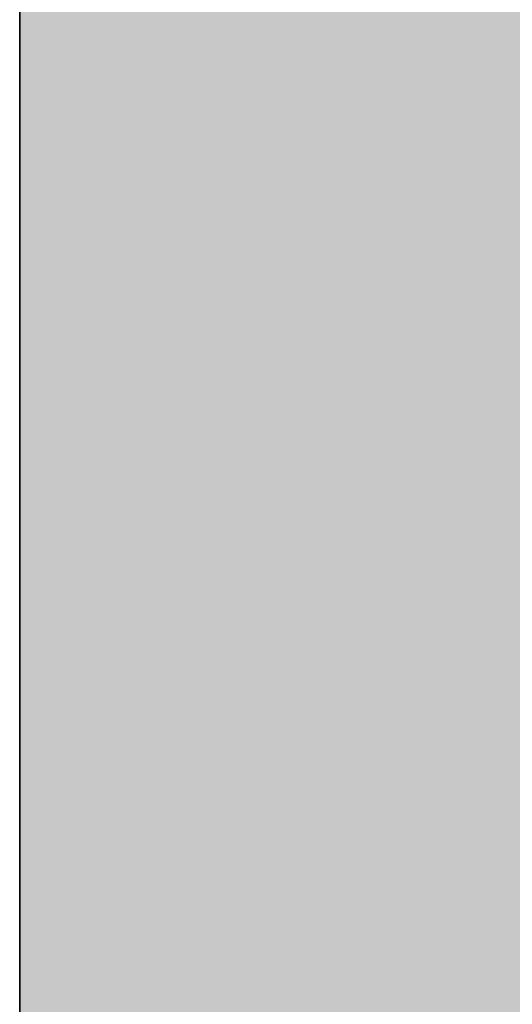
# Model space of a CAD drawing. Units: inches. Extents: x 2091 to 2899, y 967 to 2217.
# Tile 163 of 256: x 2203.143603 to 2203.144443, y 1152.248741 to 1152.250422. Entities that reach past the tile are written whole.
import ezdxf

# ---------------------------------------------------------------- set-up
doc = ezdxf.new("R2010")
doc.units = ezdxf.units.IN
doc.layers.add('A-WALL-PATT', color=141, linetype='Continuous', lineweight=13, true_color=0xadddf7)
doc.layers.add('C-PROP', color=7, linetype='Continuous', lineweight=35)

msp = doc.modelspace()

# ---------------------------------------------------------------- hatches: boundary and pattern name
at = {"layer": 'A-WALL-PATT'}
h = msp.add_hatch(color=256, dxfattribs=at)
h.dxf.hatch_style = 1
h.paths.add_polyline_path([(2803.1436027, 2050.9190588), (2203.1436027, 2050.9190588), (2203.1436027, 1090.9190588), (2803.1436027, 1090.9190588)])
h.paths.add_polyline_path([(2635.7988501, 1147.5404649), (2674.5240524, 1147.5404649, 0.376086), (2678.5296653, 1152.8802017), (2678.5296653, 1159.5564734, 0.333335), (2674.524319, 1163.561846), (2674.524319, 1163.5618504), (2674.524319, 1192.9343904), (2635.8059707, 1192.9343904), (2597.0876225, 1192.9343904), (2597.0876225, 1163.561846, 0.333335), (2593.0822761, 1159.5564734), (2593.0822761, 1152.8802017, 0.376086), (2597.087889, 1147.5404649)], flags=0)
h.paths.add_polyline_path([(2436.0104329, 1278.2407784, 0.000483), (2435.9526433, 1278.215027, -0.001328), (2435.9356253, 1278.1116934, -0.001711), (2436.1164401, 1278.0407583, 0.002185)], flags=0)
h.paths.add_polyline_path([(2794.1436027, 1143.4190588), (2794.1436027, 1347.4190588), (2543.3701706, 1347.4190588), (2543.3701706, 1351.9190588), (2794.1436027, 1351.9190588), (2794.1436027, 1392.7135549), (2793.9473982, 1392.7135549), (2793.9473982, 1473.5368999), (2794.1436027, 1473.5368999), (2794.1436027, 1531.9190588), (2650.1436027, 1531.9190588), (2650.1436027, 1536.4190588), (2794.1436027, 1536.4190588), (2794.1436027, 1692.4190588), (2609.3756095, 1692.4190588), (2609.3756095, 1644.4190588), (2604.8756095, 1644.4190588), (2604.8756095, 1744.9190588), (2609.3756095, 1744.9190588), (2609.3756095, 1696.9190588), (2794.1436027, 1696.9190588), (2794.1436027, 1780.9190588), (2609.6436027, 1780.9190588), (2493.8756095, 1780.9190588), (2493.8756095, 1785.4190588), (2609.6436027, 1785.4190588), (2794.1436027, 1785.4190588), (2794.1436027, 1847.9388214), (2793.9512217, 1847.9388214), (2793.9512217, 1928.7621663), (2794.1436027, 1928.7621663), (2794.1436027, 1941.4190588), (2614.1436027, 1941.4190588), (2614.1436027, 1821.4190588), (2609.6436027, 1821.4190588), (2609.6436027, 1941.4190588), (2392.1436027, 1941.4190588), (2392.1436027, 1819.9190588), (2387.6436027, 1819.9190588), (2387.6436027, 1941.4190588), (2212.1436027, 1941.4190588), (2212.1436027, 1783.9190588), (2392.1436027, 1783.9190588), (2392.1436027, 1780.9190588), (2212.1436027, 1780.9190588), (2212.1436027, 1629.4190588), (2387.6436027, 1629.4190588), (2387.6436027, 1744.9190588), (2392.1436027, 1744.9190588), (2392.1436027, 1627.9190588), (2317.1436027, 1627.9190588), (2317.1436027, 1551.4190588), (2317.1436027, 1536.4190588), (2459.3835909, 1536.4190588), (2459.3835909, 1602.3964802), (2463.8835909, 1602.3964802), (2463.8835909, 1531.9190588), (2456.6436027, 1531.9190588), (2456.6436027, 1529.9190588), (2452.1436027, 1529.9190588), (2452.1436027, 1531.9190588), (2312.6436027, 1531.9190588), (2312.6436027, 1551.4190588), (2306.1436027, 1551.4190588), (2306.1436027, 1555.9190588), (2308.1436027, 1555.9190588), (2308.1436027, 1551.4190588), (2312.6436027, 1551.4190588), (2312.6436027, 1627.9190588), (2212.1436027, 1627.9190588), (2212.1436027, 1555.9190588), (2270.1436027, 1555.9190588), (2270.1436027, 1551.4190588), (2212.1436027, 1551.4190588), (2212.1436027, 1351.9190588), (2272.1436027, 1351.9190588), (2272.1436027, 1347.4190588), (2212.1436027, 1347.4190588), (2212.1436027, 1275.4190588), (2308.1436027, 1275.4190588), (2308.1436027, 1351.9190588), (2452.1436027, 1351.9190588), (2452.1436027, 1493.9190588), (2456.6436027, 1493.9190588), (2456.6436027, 1347.4190588), (2312.6436027, 1347.4190588), (2312.6436027, 1270.9190588), (2212.1436027, 1270.9190588), (2212.1436027, 1099.9190588), (2281.2375229, 1099.9190588), (2282.8710413, 1110.9138034), (2282.0083413, 1116.9966034), (2278.5577413, 1121.4204034), (2268.2056413, 1128.0562034), (2272.0876413, 1128.0562034), (2273.8129413, 1131.9270034), (2279.4203413, 1134.6919034), (2285.0278413, 1135.2449034), (2287.6158413, 1137.4568034), (2288.0471413, 1138.0098034), (2289.3411413, 1140.7747034), (2291.0665413, 1139.6687034), (2292.3605413, 1135.2449034), (2295.3798413, 1136.9038034), (2296.2425413, 1135.7979034), (2297.1052413, 1133.0330034), (2300.1246413, 1138.0098034), (2303.1439413, 1138.0098034), (2304.4379413, 1135.7979034), (2303.1439413, 1133.5860034), (2306.5946413, 1134.6919034), (2307.8887413, 1133.0330034), (2310.9080413, 1135.2449034), (2313.9274413, 1134.1389034), (2315.6268599, 1132.4271023), (2308.3200413, 1117.5496034), (2290.2038413, 1109.8079034), (2288.9098413, 1103.1721034), (2289.2723086, 1099.9190588), (2434.9182274, 1099.9190588), (2431.5932274, 1124.7880588), (2429.9302274, 1169.5530588), (2430.9271848, 1240.5196942), (2435.6589255, 1238.1861258), (2437.1352274, 1196.5540588), (2438.7982274, 1143.9730588), (2442.6782274, 1111.9980588), (2446.5582274, 1099.9190588), (2794.1436027, 1099.9190588), (2794.1436027, 1138.9190588), (2548.0324471, 1138.9190588), (2548.0324471, 1143.4190588), (2548.0324471, 1148.8190588), (2546.6684571, 1148.0315588), (2528.6856919, 1179.1786218, 0.256256), (2512.0324471, 1148.8190588), (2512.0324471, 1143.4190588), (2512.0324471, 1138.9190588), (2507.5324471, 1138.9190588), (2507.5324471, 1143.4190588), (2507.5324471, 1148.8190588, 0.256256), (2490.8792023, 1179.1786218), (2472.8964371, 1148.0315588), (2471.5324471, 1148.8190588), (2471.5324471, 1143.4190588), (2467.0324471, 1143.4190588), (2467.0324471, 1269.9457858, 0.039061), (2460.9099871, 1273.5800588), (2467.0324471, 1273.5800588), (2467.0324471, 1286.3253638, 0.014511), (2465.2161944, 1286.7619052), (2467.0324471, 1287.0525761), (2467.0324471, 1323.4190588), (2471.5324471, 1323.4190588), (2471.5324471, 1148.8190588), (2489.5324471, 1179.9959734), (2490.8964371, 1179.2084734), (2490.8792023, 1179.1786218, -0.256256), (2507.5324471, 1148.8190588), (2507.5324471, 1143.4190588), (2512.0324471, 1143.4190588), (2512.0324471, 1148.8190588, -0.256256), (2528.6856919, 1179.1786218), (2528.6684571, 1179.2084734), (2530.0324471, 1179.9959734), (2548.0324471, 1148.8190588), (2548.0324471, 1143.4190588)], flags=16)
h.paths.add_polyline_path([(2607.7685461, 1200.9450832), (2607.7685461, 1265.0306251), (2597.0876225, 1281.0520106), (2619.7845852, 1281.0520106), (2627.795278, 1337.1268598), (2635.7988501, 1337.1268598), (2643.8166634, 1337.1268598), (2651.8273562, 1281.0520106), (2674.524319, 1281.0520106), (2663.8433953, 1265.0306251), (2663.8433953, 1200.9450832), (2635.8059707, 1200.9450832)], flags=0)
edge = h.paths.add_edge_path(flags=0)
edge.add_ellipse((13303.8962153, 1272.9987247), major_axis=(-10595.3130399, 0.0000005), ratio=0.842303870086, start_angle=0.62823721906, end_angle=0.64655409989, ccw=False)
edge.add_ellipse((2711.7004495, 1156.8526781), major_axis=(2.2197691, 0), ratio=0.84230387, start_angle=111.5352435, end_angle=180.6282372, ccw=False)
edge.add_ellipse((13303.1562922, 1272.9987246), major_axis=(-10593.0263064, 0), ratio=0.842303869544, start_angle=0.52827147182, end_angle=0.64655409706, ccw=False)
edge.add_line((2710.7645961, 1175.3332951), (2710.1299858, 1175.3332951))
edge.add_ellipse((2710.1299858, 1176.5797752), major_axis=(1.4798461, 0), ratio=0.84230387, start_angle=180, end_angle=270, ccw=False)
edge.add_line((2708.6501397, 1176.5797752), (2708.6501397, 1200.7829144))
edge.add_ellipse((2710.1299858, 1200.7829144), major_axis=(1.4798461, 0), ratio=0.84230387, start_angle=90, end_angle=180, ccw=False)
edge.add_line((2710.1299858, 1202.0293944), (2710.4650752, 1202.0293944))
edge.add_ellipse((13303.1562922, 1272.9987246), major_axis=(-10593.0263064, 0), ratio=0.842303869544, start_angle=-0.09022908859, end_angle=0.38386677879, ccw=False)
edge.add_ellipse((2710.1299858, 1290.9270308), major_axis=(-1.4798461, 0), ratio=0.84230387, start_angle=0, end_angle=90, ccw=False)
edge.add_line((2708.6501397, 1290.9270308), (2708.6501397, 1315.13017))
edge.add_ellipse((2710.1299858, 1315.13017), major_axis=(-1.4798461, 0), ratio=0.84230387, start_angle=-90, end_angle=0, ccw=False)
edge.add_line((2710.1299858, 1316.3766501), (2710.7063141, 1316.3766501))
edge.add_ellipse((3238.4017202, 1296.2895655), major_axis=(528.2339998, 0), ratio=0.84230386954, start_angle=176.349572414, end_angle=177.820049686, ccw=False)
edge.add_ellipse((2775.0630432, 1071.4506962), major_axis=(313.3077613, 0), ratio=0.84230386954, start_angle=102.125965552, end_angle=103.780528989, ccw=False)
edge.add_ellipse((2775.0630432, 1078.3056979), major_axis=(-305.3028915, 0), ratio=0.84230386955, start_angle=-79.790461003, end_angle=-77.555372706, ccw=False)
edge.add_ellipse((2695.1417666, 1541.9753825), major_axis=(-250.9602162, 0), ratio=0.84230386954, start_angle=99.256566007, end_angle=102.554932644)
edge.add_line((2741.4103262, 1334.2142554), (2747.1325454, 1337.3784768))
edge.add_ellipse((2747.5386163, 1336.8574776), major_axis=(-0.739923, 0), ratio=0.84230387, start_angle=270, end_angle=307.9331305, ccw=False)
edge.add_ellipse((2747.5386163, 1336.8574776), major_axis=(-0.739923, 0), ratio=0.84230387, start_angle=232.0668695, end_angle=270, ccw=False)
edge.add_line((2747.9446872, 1337.3784768), (2753.6669064, 1334.2142554))
edge.add_ellipse((2799.935466, 1541.9753825), major_axis=(250.9602162, 0), ratio=0.84230386954, start_angle=257.445067356, end_angle=260.743433993)
edge.add_ellipse((2720.0141894, 1078.3056979), major_axis=(305.3028915, 0), ratio=0.84230386954, start_angle=77.555372707, end_angle=79.790461003, ccw=False)
edge.add_ellipse((2720.0141894, 1071.4506962), major_axis=(-313.3077613, 0), ratio=0.84230386954, start_angle=256.219471011, end_angle=257.874034448, ccw=False)
edge.add_ellipse((2256.6755124, 1296.2895655), major_axis=(-528.2339998, 0), ratio=0.84230386954, start_angle=182.179950314, end_angle=183.650427586, ccw=False)
edge.add_line((2784.3709184, 1316.3766501), (2784.9472468, 1316.3766501))
edge.add_ellipse((2784.9472468, 1315.13017), major_axis=(1.4798461, 0), ratio=0.84230387, start_angle=0, end_angle=90, ccw=False)
edge.add_line((2786.4270928, 1315.13017), (2786.4270928, 1290.9270308))
edge.add_ellipse((2784.9472468, 1290.9270308), major_axis=(1.4798461, 0), ratio=0.84230387, start_angle=270, end_angle=360, ccw=False)
edge.add_ellipse((-7808.0790596, 1272.9987246), major_axis=(10593.0263063, 0), ratio=0.842303869544, start_angle=-0.38386677879, end_angle=0.09022908859, ccw=False)
edge.add_line((2784.6121574, 1202.0293944), (2784.9472468, 1202.0293944))
edge.add_ellipse((2784.9472468, 1200.7829144), major_axis=(1.4798461, 0), ratio=0.84230387, start_angle=0, end_angle=90, ccw=False)
edge.add_line((2786.4270928, 1200.7829144), (2786.4270928, 1176.5797752))
edge.add_ellipse((2784.9472468, 1176.5797752), major_axis=(-1.4798461, 0), ratio=0.84230387, start_angle=90, end_angle=180, ccw=False)
edge.add_line((2784.9472468, 1175.3332951), (2784.3126365, 1175.3332951))
edge.add_ellipse((-7808.0790596, 1272.9987246), major_axis=(10593.0263063, 0), ratio=0.842303869544, start_angle=-0.61864319632, end_angle=-0.52827147182, ccw=False)
edge.add_ellipse((2783.3767831, 1156.8526781), major_axis=(-2.2197691, 0), ratio=0.84230387, start_angle=179.3717628, end_angle=248.4647566, ccw=False)
edge.add_ellipse((-7808.8189826, 1272.9987246), major_axis=(-10595.3130398, 0.0000036), ratio=0.842303865762, start_angle=179.3534459226, end_angle=179.37176280343, ccw=False)
edge.add_ellipse((2780.2973026, 1153.500793), major_axis=(-5.2464256, 0), ratio=0.84230387, start_angle=90, end_angle=179.3534459, ccw=False)
edge.add_line((2780.2973026, 1149.0817084), (2714.77993, 1149.0817084))
edge.add_ellipse((2714.77993, 1153.500793), major_axis=(5.2464256, 0), ratio=0.84230387, start_angle=180.6465541, end_angle=270, ccw=False)
edge = h.paths.add_edge_path(flags=0)
edge.add_line((2718.1873674, 1151.0078329), (2718.1873674, 1170.4723638))
edge.add_ellipse((2721.1470595, 1170.4723638), major_axis=(-2.9596921, 0), ratio=0.84230387, start_angle=-90, end_angle=0, ccw=False)
edge.add_line((2721.1470595, 1172.965324), (2773.9301731, 1172.965324))
edge.add_ellipse((2773.9301731, 1170.4723638), major_axis=(-2.9596921, 0), ratio=0.84230387, start_angle=180, end_angle=270, ccw=False)
edge.add_line((2776.8898652, 1170.4723638), (2776.8898652, 1151.0078329))
edge.add_line((2776.8898652, 1151.0078329), (2718.1873674, 1151.0078329))
edge = h.paths.add_edge_path(flags=0)
edge.add_line((2718.1873674, 1180.2341502), (2718.1873674, 1199.0578342))
edge.add_ellipse((2747.5386163, 1320.3986402), major_axis=(147.0179239, 0), ratio=0.84230386954, start_angle=256.40186531, end_angle=283.59813469)
edge.add_line((2776.8898652, 1199.0578342), (2776.8898652, 1180.2341502))
edge.add_ellipse((2747.5386163, 1301.5749562), major_axis=(147.0179239, 0), ratio=0.84230386954, start_angle=256.40186531, end_angle=283.59813469, ccw=False)
edge = h.paths.add_edge_path(flags=0)
edge.add_ellipse((13303.1562922, 1272.9987246), major_axis=(-10591.5464603, 0), ratio=0.842303869555, start_angle=0.05559431352, end_angle=0.37776419393, ccw=False)
edge.add_line((2711.6168595, 1262.7217103), (2715.6674076, 1249.4953957))
edge.add_ellipse((6413.8919626, 1241.691919), major_axis=(-3698.2361592, 0), ratio=0.842303869547, start_angle=-0.120897369, end_angle=0.3640763489)
edge.add_line((2715.7610383, 1218.1924547), (2711.9343065, 1203.167361))
edge = h.paths.add_edge_path(flags=0)
edge.add_line((2718.1873674, 1251.074566), (2716.0024854, 1267.4504351))
edge.add_ellipse((2742.1511746, 1202.1895399), major_axis=(81.7725845, 0), ratio=0.8423038695, start_angle=94.277420963, end_angle=111.834953797, ccw=False)
edge.add_line((2737.0097482, 1270.9306255), (2758.0674844, 1270.9306255))
edge.add_ellipse((2752.926058, 1202.1895399), major_axis=(81.7725845, 0), ratio=0.8423038695, start_angle=68.165046203, end_angle=85.722579037, ccw=False)
edge.add_line((2779.0747472, 1267.4504351), (2776.8898652, 1251.074566))
edge.add_ellipse((2750.3380588, 1187.8853558), major_axis=(79.5796641, 0), ratio=0.8423038695, start_angle=67.208085122, end_angle=85.129930403)
edge.add_line((2756.0346562, 1254.7436557), (2739.0425764, 1254.7436557))
edge.add_ellipse((2744.7391738, 1187.8853558), major_axis=(79.5796641, 0), ratio=0.8423038695, start_angle=94.870069597, end_angle=112.791914878)
edge = h.paths.add_edge_path(flags=0)
edge.add_line((2783.1429261, 1203.167361), (2779.3161943, 1218.1924547))
edge.add_ellipse((-918.81473, 1241.691919), major_axis=(3698.2361592, 0), ratio=0.842303869546, start_angle=-0.3640763489, end_angle=0.120897369)
edge.add_line((2779.409825, 1249.4953957), (2783.4603731, 1262.7217103))
edge.add_ellipse((-7808.0790596, 1272.9987246), major_axis=(-10591.5464603, 0), ratio=0.84230386954, start_angle=179.6222358061, end_angle=179.94440568651, ccw=False)
edge = h.paths.add_edge_path(flags=0)
edge.add_ellipse((2734.2008921, 1286.6904402), major_axis=(-0.3566086, 6.3400775), ratio=0.603833576, start_angle=89.00201428, end_angle=253.65740805, ccw=False)
edge.add_line((2730.3690013, 1286.5418057), (2730.3690013, 1301.3519803))
edge.add_line((2730.3690013, 1301.3519803), (2735.9133107, 1305.2148028))
edge.add_ellipse((2736.3849168, 1304.7345612), major_axis=(0.739923, 0), ratio=0.84230387, start_angle=90, end_angle=134.4802109, ccw=False)
edge.add_line((2736.3849168, 1305.3578013), (2738.0327829, 1305.3578013))
edge.add_line((2738.0327829, 1305.3578013), (2738.0327829, 1307.7079274))
edge.add_ellipse((2794.201642, 1307.7079274), major_axis=(56.168859, 0), ratio=0.8423038695, start_angle=150.5614304, end_angle=180, ccw=False)
edge.add_ellipse((2700.8755906, 1307.7079274), major_axis=(-56.168859, 0), ratio=0.8423038695, start_angle=180, end_angle=209.4385696, ccw=False)
edge.add_line((2757.0444497, 1307.7079274), (2757.0444497, 1305.3578013))
edge.add_line((2757.0444497, 1305.3578013), (2758.6923157, 1305.3578013))
edge.add_ellipse((2758.6923157, 1304.7345612), major_axis=(-0.739923, 0), ratio=0.84230387, start_angle=225.5197891, end_angle=270, ccw=False)
edge.add_line((2759.1639219, 1305.2148028), (2764.7082312, 1301.3519803))
edge.add_line((2764.7082312, 1301.3519803), (2764.7082312, 1286.5418057))
edge.add_ellipse((2760.8763405, 1286.6904402), major_axis=(0.3566086, 6.3400775), ratio=0.603833576, start_angle=106.34259195, end_angle=270.99798572, ccw=False)
edge.add_line((2757.0444497, 1285.7970896), (2757.0444497, 1307.7079274))
edge.add_ellipse((2700.8755906, 1307.7079274), major_axis=(-56.168859, 0), ratio=0.8423038695, start_angle=180, end_angle=209.4385696)
edge.add_ellipse((2794.201642, 1307.7079274), major_axis=(56.168859, 0), ratio=0.8423038695, start_angle=150.5614304, end_angle=180)
edge.add_line((2738.0327829, 1307.7079274), (2738.0327829, 1285.7970896))
h.paths.add_polyline_path([(2417.8122727, 1104.449704), (2413.4922727, 1102.529704), (2410.6122727, 1103.969704), (2409.1722727, 1106.369704), (2407.2522727, 1107.329704), (2406.2922727, 1109.729704), (2405.3322727, 1114.049704), (2405.3322727, 1117.889704), (2406.2922727, 1120.129704), (2407.2522727, 1119.809704), (2408.8483218, 1118.3276585), (2410.1739451, 1119.4241703), (2410.2112727, 1120.405704), (2411.0407305, 1121.4190541), (2410.6992727, 1119.858704), (2410.1739451, 1119.4241703), (2410.0884515, 1117.1761095), (2411.1328361, 1116.2063237), (2413.9722727, 1119.329704), (2416.8522727, 1120.769704), (2416.8697209, 1120.7987842), (2417.0350713, 1119.4051162), (2417.8962134, 1118.1433844), (2418.2922727, 1118.369704), (2419.5444467, 1120.0392692), (2419.3609153, 1118.387487), (2419.0321078, 1119.3561507), (2418.3989394, 1118.5119262), (2419.2522727, 1114.529704), (2418.7940909, 1107.1987949)], flags=0)
h.paths.add_polyline_path([(2508.8701706, 1347.4190588), (2508.3701706, 1347.4190588), (2508.3701706, 1351.9190588), (2508.8701706, 1351.9190588)], flags=0)
h.paths.add_polyline_path([(2473.3701706, 1347.4190588), (2472.3701706, 1347.4190588), (2467.8701706, 1347.4190588), (2467.8701706, 1455.4190588), (2472.3701706, 1455.4190588), (2472.3701706, 1352.4190588), (2473.3701706, 1352.4190588)], flags=0)
h.paths.add_polyline_path([(2352.106244, 1217.4461971), (2349.226244, 1218.8861971), (2347.786244, 1221.2861971), (2345.866244, 1222.2461971), (2344.906244, 1224.6461971), (2343.946244, 1228.9661971), (2343.946244, 1232.8061971), (2344.906244, 1235.0461971), (2345.866244, 1234.7261971), (2347.4622931, 1233.2441515), (2348.7879164, 1234.3406634), (2348.825244, 1235.3221971), (2349.6547018, 1236.3355471), (2349.313244, 1234.7751971), (2348.7879164, 1234.3406634), (2348.7024228, 1232.0926025), (2349.7468074, 1231.1228168), (2352.586244, 1234.2461971), (2355.466244, 1235.6861971), (2355.4836921, 1235.7152773), (2355.6490426, 1234.3216093), (2356.5101846, 1233.0598774), (2356.906244, 1233.2861971), (2358.1584179, 1234.9557623), (2357.9748866, 1233.3039801), (2357.6460791, 1234.2726438), (2357.0129107, 1233.4284193), (2357.866244, 1229.4461971), (2357.4080622, 1222.115288), (2356.426244, 1219.3661971)], flags=0)
h.paths.add_polyline_path([(2348.2967999, 1112.2244204), (2347.0137999, 1112.3104204), (2345.5297999, 1114.1274204), (2345.7317999, 1115.8584204), (2346.8117999, 1116.9824204), (2346.8117999, 1114.6464204), (2345.8667999, 1114.2144204), (2346.8797999, 1114.3004204)], flags=0)
h.paths.add_polyline_path([(2347.0137999, 1110.9264204), (2346.2717999, 1110.4934204), (2346.6097999, 1111.1864204)], flags=0)
h.paths.add_polyline_path([(2345.8667999, 1118.1944204), (2345.5297999, 1117.3294204), (2343.7077999, 1118.0214204), (2344.3827999, 1118.6264204)], flags=0)
h.paths.add_polyline_path([(2346.6767999, 1109.2824204), (2346.0697999, 1108.0714204), (2345.8667999, 1110.0614204)], flags=0)
h.paths.add_polyline_path([(2345.0567999, 1119.7514204), (2343.6397999, 1119.7514204), (2343.9777999, 1121.1354204)], flags=0)
h.paths.add_polyline_path([(2345.2597999, 1116.5504204), (2345.1247999, 1115.8584204), (2344.9217999, 1115.6854204), (2344.7197999, 1116.3774204)], flags=0)
h.paths.add_polyline_path([(2345.6647999, 1112.3104204), (2345.4617999, 1111.5324204), (2344.0447999, 1111.9644204), (2344.6517999, 1112.5704204)], flags=0)
h.paths.add_polyline_path([(2345.1917999, 1113.3494204), (2344.4497999, 1113.8684204), (2344.7197999, 1114.3874204)], flags=0)
h.paths.add_polyline_path([(2344.6517999, 1116.8094204), (2344.1797999, 1115.6854204), (2344.6517999, 1115.3394204), (2343.9097999, 1114.9064204), (2343.0327999, 1115.9444204), (2343.6397999, 1116.4634204)], flags=0)
h.paths.add_polyline_path([(2345.8667999, 1106.6864204), (2344.9897999, 1105.5624204), (2344.5167999, 1106.6004204)], flags=0)
h.paths.add_polyline_path([(2344.8547999, 1110.0614204), (2344.5167999, 1109.2824204), (2344.1127999, 1109.7154204)], flags=0)
h.paths.add_polyline_path([(2344.0447999, 1113.5224204), (2343.4377999, 1113.0894204), (2342.7627999, 1113.9544204)], flags=0)
h.paths.add_polyline_path([(2344.3147999, 1111.0124204), (2342.9647999, 1110.3204204), (2342.9647999, 1111.0994204)], flags=0)
h.paths.add_polyline_path([(2345.1247999, 1104.6974204), (2344.5847999, 1103.7454204), (2344.4497999, 1104.2644204)], flags=0)
h.paths.add_polyline_path([(2342.8297999, 1121.2224204), (2341.7497999, 1120.5304204), (2340.5357999, 1121.0494204), (2340.1307999, 1121.8284204), (2340.6707999, 1122.9524204), (2341.1427999, 1121.8284204), (2341.6147999, 1122.0014204)], flags=0)
h.paths.add_polyline_path([(2342.9647999, 1119.7514204), (2343.0327999, 1118.4534204), (2342.0877999, 1118.0214204), (2342.0197999, 1119.4914204)], flags=0)
h.paths.add_polyline_path([(2342.6947999, 1116.8964204), (2341.9527999, 1116.6364204), (2342.0197999, 1117.3294204)], flags=0)
h.paths.add_polyline_path([(2343.0327999, 1112.2244204), (2342.0197999, 1111.7914204), (2341.5477999, 1112.2244204), (2342.3577999, 1113.3494204)], flags=0)
h.paths.add_polyline_path([(2343.7747999, 1104.4374204), (2342.6277999, 1102.8804204), (2342.6947999, 1104.6104204), (2343.4377999, 1105.1294204)], flags=0)
h.paths.add_polyline_path([(2342.0197999, 1115.0794204), (2340.8057999, 1115.5124204), (2340.9407999, 1116.3774204)], flags=0)
h.paths.add_polyline_path([(2341.4807999, 1120.0974204), (2341.4807999, 1119.4054204), (2341.0757999, 1119.5784204), (2341.1427999, 1120.0974204)], flags=0)
h.paths.add_polyline_path([(2341.8177999, 1114.4734204), (2340.9407999, 1113.0894204), (2340.8057999, 1114.5604204)], flags=0)
h.paths.add_polyline_path([(2341.1427999, 1118.5404204), (2340.9407999, 1116.9824204), (2339.0507999, 1117.6754204), (2339.0507999, 1118.6264204)], flags=0)
h.paths.add_polyline_path([(2342.6947999, 1101.6684204), (2341.9527999, 1101.8414204), (2342.5597999, 1102.3614204)], flags=0)
h.paths.add_polyline_path([(2340.3327999, 1119.6654204), (2338.4437999, 1119.5784204), (2337.9037999, 1120.3574204), (2339.6577999, 1120.6164204)], flags=0)
h.paths.add_polyline_path([(2340.3327999, 1115.3394204), (2340.0627999, 1113.6954204), (2339.3877999, 1115.3394204)], flags=0)
h.paths.add_polyline_path([(2341.8177999, 1103.8314204), (2341.5477999, 1102.8804204), (2341.1427999, 1103.6584204)], flags=0)
h.paths.add_polyline_path([(2339.0507999, 1122.8664204), (2337.2957999, 1121.8284204), (2337.0937999, 1123.1254204), (2337.7687999, 1123.8184204)], flags=0)
h.paths.add_polyline_path([(2339.1177999, 1121.7414204), (2338.8477999, 1121.2224204), (2338.1737999, 1121.0494204), (2338.3757999, 1121.5684204)], flags=0)
h.paths.add_polyline_path([(2339.1857999, 1119.3194204), (2338.6457999, 1118.7134204), (2338.2407999, 1118.1074204), (2338.2407999, 1118.8864204)], flags=0)
h.paths.add_polyline_path([(2341.1427999, 1101.9284204), (2340.6027999, 1101.2364204), (2340.0627999, 1101.8414204), (2340.6027999, 1102.3614204)], flags=0)
h.paths.add_polyline_path([(2337.6337999, 1117.7614204), (2336.6207999, 1118.2804204), (2337.2957999, 1118.9724204)], flags=0)
h.paths.add_polyline_path([(2336.8237999, 1119.5784204), (2334.7987999, 1118.9724204), (2335.2037999, 1120.3574204), (2336.5537999, 1120.8764204)], flags=0)
h.paths.add_polyline_path([(2339.1177999, 1100.4574204), (2337.3637999, 1100.5434204), (2336.7557999, 1101.2364204)], flags=0)
h.paths.add_polyline_path([(2336.3507999, 1122.4334204), (2336.0137999, 1121.9144204), (2334.9337999, 1122.4334204), (2334.5287999, 1123.4714204), (2335.7437999, 1122.7794204)], flags=0)
h.paths.add_polyline_path([(2334.7317999, 1120.8764204), (2334.2587999, 1120.3574204), (2334.0567999, 1120.7894204), (2334.5967999, 1121.3084204)], flags=0)
h.paths.add_polyline_path([(2334.4617999, 1122.1744204), (2332.5717999, 1121.3084204), (2331.3567999, 1122.1744204), (2332.0997999, 1122.8664204)], flags=0)
h.paths.add_polyline_path([(2334.2587999, 1118.5404204), (2333.3817999, 1118.4534204), (2333.6517999, 1119.3194204)], flags=0)
h.paths.add_polyline_path([(2335.5417999, 1102.2744204), (2334.1917999, 1102.6204204), (2335.2717999, 1103.3124204)], flags=0)
h.paths.add_polyline_path([(2332.7067999, 1119.6654204), (2331.6947999, 1120.4434204), (2332.5047999, 1120.7894204)], flags=0)
h.paths.add_polyline_path([(2334.7317999, 1101.1494204), (2333.5167999, 1101.5824204), (2333.9887999, 1101.7554204)], flags=0)
h.paths.add_polyline_path([(2332.6397999, 1116.6364204), (2331.0867999, 1116.2904204), (2331.9647999, 1118.1944204)], flags=0)
h.paths.add_polyline_path([(2330.7497999, 1121.5684204), (2330.2767999, 1120.2704204), (2328.5227999, 1119.3194204), (2328.9947999, 1121.0494204)], flags=0)
h.paths.add_polyline_path([(2330.7497999, 1118.6264204), (2330.0077999, 1117.5024204), (2329.8727999, 1118.0214204)], flags=0)
h.paths.add_polyline_path([(2332.0997999, 1102.3614204), (2330.5467999, 1102.0144204), (2331.6947999, 1102.9664204)], flags=0)
h.paths.add_polyline_path([(2329.5347999, 1113.6084204), (2329.0627999, 1112.3104204), (2328.5897999, 1113.3494204)], flags=0)
h.paths.add_polyline_path([(2328.3877999, 1117.8484204), (2327.5097999, 1116.5504204), (2327.1727999, 1117.7614204)], flags=0)
h.paths.add_polyline_path([(2329.7377999, 1106.5134204), (2329.5347999, 1105.3024204), (2328.2527999, 1106.0814204)], flags=0)
h.paths.add_polyline_path([(2328.6577999, 1114.3874204), (2328.0497999, 1114.1274204), (2328.3197999, 1114.9064204)], flags=0)
h.paths.add_polyline_path([(2328.3197999, 1112.2244204), (2327.1057999, 1112.1374204), (2326.7007999, 1112.6564204)], flags=0)
h.paths.add_polyline_path([(2326.9027999, 1115.2524204), (2326.7007999, 1114.1274204), (2325.2157999, 1113.6084204), (2326.0927999, 1115.3394204)], flags=0)
h.paths.add_polyline_path([(2326.6327999, 1108.3304204), (2326.0927999, 1107.3794204), (2325.8907999, 1108.5034204), (2326.4977999, 1109.1094204)], flags=0)
h.paths.add_polyline_path([(2615.1436027, 1531.9190588), (2609.6436027, 1531.9190588), (2609.6436027, 1620.4190588), (2614.1436027, 1620.4190588), (2614.1436027, 1536.4190588), (2615.1436027, 1536.4190588)], flags=0)
h.paths.add_polyline_path([(2545.1436027, 1563.4190588), (2464.1436027, 1563.4190588), (2464.1436027, 1632.4190588), (2509.1436027, 1632.4190588), (2509.1436027, 1627.9190588), (2509.1436027, 1603.9190588), (2468.6436027, 1603.9190588), (2468.6436027, 1567.9190588), (2540.6436027, 1567.9190588), (2540.6436027, 1591.9190588), (2545.1436027, 1591.9190588)], flags=0)
h.paths.add_polyline_path([(2388.9690483, 1549.985735), (2357.4341811, 1549.985735), (2357.4341811, 1623.3607783), (2399.3627772, 1623.3607783), (2435.6894654, 1623.3607783), (2435.5925469, 1602.5592734), (2435.5925469, 1602.3964802), (2388.9690483, 1602.3964802)], flags=0)
h.paths.add_polyline_path([(2388.8806282, 1555.8091511), (2374.9044295, 1555.8091511), (2374.9044295, 1600.5715641), (2374.9044295, 1615.4576454), (2406.3508766, 1615.4576454), (2406.3508766, 1618.9394309), (2412.1742927, 1615.4576454), (2406.3508766, 1611.9758599), (2406.3508766, 1615.4576454), (2388.8806282, 1615.4576454)], flags=0)
h.paths.add_polyline_path([(2568.8756095, 1644.4190588), (2453.3756095, 1644.4190588), (2453.3756095, 1785.4190588), (2457.8756095, 1785.4190588), (2457.8756095, 1648.9190588), (2568.8756095, 1648.9190588)], flags=0)
h.paths.add_polyline_path([(2212.1436027, 1945.9190588), (2212.1436027, 2041.9190588), (2794.1436027, 2041.9190588), (2794.1436027, 1945.9190588)], flags=16)
h.paths.add_polyline_path([(2271.0827276, 1964.3172377), (2776.852968, 1964.3172377), (2776.852968, 2037.1696226), (2271.0827276, 2037.1696226)], flags=8)
h.paths.add_polyline_path([(2380.6492852, 1536.8241435), (2461.0408087, 1536.8241435), (2461.0408087, 1554.6525871), (2380.6492852, 1554.6525871)], flags=8)
h.paths.add_polyline_path([(2240.7557092, 1609.7254508), (2309.1858294, 1609.7254508), (2309.1858294, 1617.6982037), (2240.7557092, 1617.6982037)], flags=8)
h.paths.add_polyline_path([(2212.6772554, 1313.5041021), (2282.5915203, 1313.5041021), (2282.5915203, 1322.7452389), (2212.6772554, 1322.7452389)], flags=8)
h.paths.add_polyline_path([(2457.111976, 1114.778574), (2558.4815807, 1114.778574), (2558.4815807, 1142.2196823), (2457.111976, 1142.2196823)], flags=8)
h.paths.add_polyline_path([(2473.4423372, 1273.0100672), (2604.6412257, 1273.0100672), (2604.6412257, 1318.3469349), (2473.4423372, 1318.3469349)], flags=8)
h.paths.add_polyline_path([(2638.8763024, 1626.9774316), (2684.2503675, 1627.9767377), (2684.0384825, 1637.5974944), (2638.6644174, 1636.5981884)], flags=8)
h.paths.add_polyline_path([(2537.5905538, 1453.7934466), (2628.3895472, 1453.7934466), (2628.3895472, 1475.3448114), (2537.5905538, 1475.3448114)], flags=8)
h.paths.add_polyline_path([(2504.1376376, 1714.6323972), (2554.6471875, 1714.6323972), (2554.6471875, 1730.2377115), (2504.1376376, 1730.2377115)], flags=8)
h.paths.add_polyline_path([(2487.5011806, 1575.6518716), (2535.0971214, 1575.6518716), (2535.0971214, 1598.3776456), (2487.5011806, 1598.3776456)], flags=8)
h.paths.add_polyline_path([(2709.0994004, 1735.7102784), (2740.0166009, 1735.7102784), (2740.0166009, 1749.9376406), (2709.0994004, 1749.9376406)], flags=8)
h.paths.add_polyline_path([(2442.4384239, 1792.1716575), (2564.7288353, 1792.1716575), (2564.7288353, 1842.0001626), (2442.4384239, 1842.0001626)], flags=8)
h.paths.add_polyline_path([(2655.8158012, 1809.6440763), (2789.5201425, 1806.6937963), (2790.0849768, 1832.2916379), (2656.3806355, 1835.2419179)], flags=8)
h.paths.add_polyline_path([(2234.8426972, 1797.7201432), (2368.5928512, 1794.7688523), (2369.1607182, 1820.504132), (2235.4105642, 1823.4554229)], flags=8)
h.paths.add_polyline_path([(2245.1384659, 1644.0063348), (2398.4277329, 1640.6238997), (2398.9948417, 1666.3248199), (2245.7055747, 1669.7072549)], flags=8)
h.paths.add_polyline_path([(2306.1428474, 1431.1685186), (2413.7683138, 1428.7936873), (2414.3331481, 1454.3915289), (2306.7076817, 1456.7663602)], flags=8)
h.paths.add_polyline_path([(2306.834582, 1458.2331447), (2393.3804836, 1456.3234487), (2393.9328082, 1481.3543583), (2307.3869066, 1483.2640542)], flags=8)

# ---------------------------------------------------------------- linework, layer by layer
at = {"layer": 'C-PROP'}
msp.add_lwpolyline([(2203.1436027, 2050.9190588), (2803.1436027, 2050.9190588), (2803.1436027, 1090.9190588), (2203.1436027, 1090.9190588)], close=True, dxfattribs=at)

doc.saveas('drawing.dxf')
